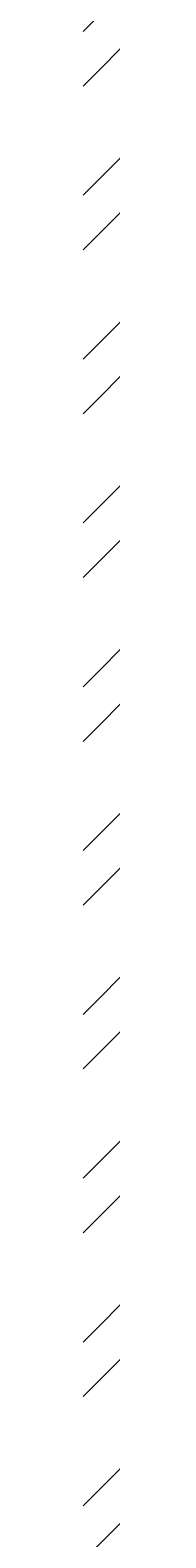
# Model space of a CAD drawing. Units: inches. Extents: x 1962 to 2771, y 1245 to 2660.
# Tile 106 of 114: x 2372 to 2374, y 2180 to 2304. Entities that reach past the tile are written whole.
import ezdxf

# ---------------------------------------------------------------- set-up
doc = ezdxf.new("R2010")
doc.units = ezdxf.units.IN
doc.layers.add('A-ANNO-DIMS', color=2, linetype='Continuous', lineweight=18)
doc.layers.add('A-WALL-PATT', color=252, linetype='Continuous', lineweight=13)
doc.styles.get("Standard").update_dxf_attribs({"font": 'arial.ttf'})
doc.dimstyles.get("Standard").update_dxf_attribs({"dimtxt": 0.18, "dimasz": 0.18, "dimexe": 0.18, "dimexo": 0.0625, "dimgap": 0.09, "dimtad": 0, "dimtih": 1, "dimtoh": 1, "dimdec": 4, "dimzin": 0, "dimdsep": 46, "dimtxsty": 'Standard', "dimcen": 0.09, "dimadec": 0, "dimazin": 0, "dimtfac": 1, "dimtdec": 4, "dimtofl": 0, "dimtmove": 0, "dimatfit": 3, "dimfxl": 1, "dimtolj": 1, "dimtzin": 0, "dimarcsym": 0})

# ---------------------------------------------------------------- blocks, each defined once
blk = doc.blocks.new('*D40')
at = {"layer": 'A-ANNO-DIMS', "color": 0, "lineweight": -2, "transparency": 16777216}
for p, q in [((2072.02, 2033.91), (2072.02, 2583.47)), ((2660.81, 2524.41), (2660.81, 2583.47)), ((2072.2, 2583.29), (2366.02, 2583.29)), ((2660.63, 2583.29), (2366.81, 2583.29))]:
    blk.add_line(p, q, dxfattribs=at)
at = {"layer": 'A-ANNO-DIMS', "color": 0, "transparency": 16777216}
for points in [[(2072.2, 2583.32), (2072.2, 2583.26), (2072.02, 2583.29)], [(2660.63, 2583.32), (2660.63, 2583.26), (2660.81, 2583.29)]]:
    blk.add_solid(points, dxfattribs=at)
at = {"layer": 'Defpoints', "color": 0, "transparency": 16777216}
for p in [(2660.81, 2583.29), (2660.81, 2524.34), (2072.02, 2033.84)]:
    blk.add_point(p, dxfattribs=at)
at = {"layer": 'A-ANNO-DIMS', "color": 0, "transparency": 16777216, "insert": (2366.41, 2583.29), "char_height": 0.18, "attachment_point": 5}
blk.add_mtext('\\A1;588.8', dxfattribs=at)

msp = doc.modelspace()

# ---------------------------------------------------------------- hatches: boundary and pattern name
at = {"layer": 'A-WALL-PATT'}
h = msp.add_hatch(dxfattribs=at)
h.set_pattern_fill('ANSI32', color=256)
h.paths.add_polyline_path([(2090.8074, 2467.3437), (2141.6481, 2467.3437), (2141.6481, 2469.5937), (2141.6481, 2471.8437), (2086.3074, 2471.8437), (2086.3074, 2422.5333), (2090.8074, 2422.5333)])
h.paths.add_polyline_path([(2282.7664, 2471.8437), (2204.8982, 2471.8437), (2204.8982, 2467.3437), (2234.8074, 2467.3437), (2234.8074, 2311.3437), (2228.7492, 2311.3437), (2228.7492, 2306.8437), (2234.8074, 2306.8437), (2331.9227, 2306.8437), (2331.9227, 2309.0937), (2331.9227, 2311.3437), (2239.3074, 2311.3437), (2239.3074, 2467.3437), (2282.7664, 2467.3437), (2282.7664, 2469.5937)])
h.paths.add_polyline_path([(2471.4531, 2519.8437), (2552.011, 2519.8437), (2564.3996, 2519.8437), (2564.3996, 2511.1389), (2568.8996, 2511.1389), (2568.8996, 2524.3437), (2466.9531, 2524.3437), (2466.9531, 2471.8437), (2450.0749, 2471.8437), (2446.4672, 2471.8437), (2446.4672, 2467.3437), (2450.0749, 2467.3437), (2475.9988, 2467.3437), (2475.9988, 2469.5937), (2475.9988, 2471.8437), (2471.4531, 2471.8437)])
h.paths.add_polyline_path([(2575.2231, 2469.5937), (2575.2231, 2471.8437), (2568.8996, 2471.8437), (2568.8996, 2487.1389), (2564.3996, 2487.1389), (2564.3996, 2471.8437), (2556.511, 2471.8437), (2499.2904, 2471.8437), (2499.2904, 2467.3437), (2507.8074, 2467.3437), (2507.8074, 2311.3437), (2414.863, 2311.3437), (2414.863, 2306.8437), (2512.3074, 2306.8437), (2517.0114, 2306.8437), (2517.0114, 2309.0937), (2517.0114, 2311.3437), (2512.3074, 2311.3437), (2512.3074, 2467.3437), (2575.2231, 2467.3437)])
h.paths.add_polyline_path([(2660.8074, 2471.8437), (2600.9602, 2471.8437), (2600.9602, 2467.3437), (2656.3074, 2467.3437), (2656.3074, 2432.5704), (2660.8074, 2432.5704)])
h.paths.add_polyline_path([(2660.8074, 2372.5704), (2656.3074, 2372.5704), (2656.3074, 2311.3437), (2600.276, 2311.3437), (2600.276, 2309.0937), (2600.276, 2306.8437), (2656.3074, 2306.8437), (2656.3074, 2296.2593), (2660.8074, 2296.2593)])
h.paths.add_polyline_path([(2572.3074, 2306.8437), (2577.1385, 2306.8437), (2577.1385, 2311.3437), (2551.082, 2311.3437), (2551.082, 2306.8437), (2567.8074, 2306.8437), (2567.8074, 2258.8437), (2540.0574, 2258.8437), (2540.0574, 2256.5937), (2540.0574, 2254.3437), (2567.8074, 2254.3437), (2656.3074, 2254.3437), (2656.3074, 2236.9085), (2660.8074, 2236.9085), (2660.8074, 2272.2593), (2656.3074, 2272.2593), (2656.3074, 2258.8437), (2572.3074, 2258.8437)])
h.paths.add_polyline_path([(2512.3074, 2254.3437), (2518.8716, 2254.3437), (2518.8716, 2256.5937), (2518.8716, 2258.8437), (2507.8074, 2258.8437), (2507.8074, 2177.8437), (2567.8074, 2177.8437), (2567.8074, 2172.9628), (2572.3074, 2172.9628), (2572.3074, 2177.8437), (2656.3074, 2177.8437), (2656.3074, 2166.4846), (2660.8074, 2166.4846), (2660.8074, 2200.9085), (2656.3074, 2200.9085), (2656.3074, 2182.3437), (2512.3074, 2182.3437)])
h.paths.add_polyline_path([(2656.3074, 2129.8437), (2572.3074, 2129.8437), (2572.3074, 2150.3044), (2570.0574, 2150.3044), (2567.8074, 2150.3044), (2567.8074, 2129.8437), (2507.8074, 2129.8437), (2507.8074, 2116.3027), (2510.0574, 2116.3027), (2512.3074, 2116.3027), (2512.3074, 2125.3437), (2567.8074, 2125.3437), (2572.3074, 2125.3437), (2656.3074, 2125.3437)])
h.paths.add_polyline_path([(2090.8074, 2362.5333), (2086.3074, 2362.5333), (2086.3074, 2298.6242), (2090.8074, 2298.6242), (2090.8074, 2306.8437), (2174.8074, 2306.8437), (2174.8074, 2286.4178), (2179.3074, 2286.4178), (2179.3074, 2306.8437), (2192.8641, 2306.8437), (2192.8641, 2309.0937), (2192.8641, 2311.3437), (2090.8074, 2311.3437)])
h.paths.add_polyline_path([(2209.156, 2258.8437), (2179.3074, 2258.8437), (2179.3074, 2263.2236), (2177.0574, 2263.2236), (2174.8074, 2263.2236), (2174.8074, 2258.8437), (2090.8074, 2258.8437), (2090.8074, 2274.6242), (2086.3074, 2274.6242), (2086.3074, 2238.2967), (2088.5574, 2238.2967), (2090.8074, 2238.2967), (2090.8074, 2254.3437), (2209.156, 2254.3437)])
h.paths.add_polyline_path([(2090.8074, 2177.8437), (2234.8074, 2177.8437), (2234.8074, 2173.1428), (2239.3074, 2173.1428), (2239.3074, 2258.8437), (2230.8442, 2258.8437), (2230.8442, 2256.5937), (2230.8442, 2254.3437), (2234.8074, 2254.3437), (2234.8074, 2182.3437), (2090.8074, 2182.3437), (2090.8074, 2202.2967), (2086.3074, 2202.2967), (2086.3074, 2140.0389), (2090.8074, 2140.0389)])
h.paths.add_polyline_path([(2090.8074, 2080.0389), (2086.3074, 2080.0389), (2086.3074, 2033.8437), (2090.8074, 2033.8437)], flags=17)
h.paths.add_polyline_path([(2244.9405, 2033.8437), (2239.3074, 2033.8437), (2239.3074, 2142.0665), (2237.2592, 2142.0665), (2234.8074, 2142.0665), (2234.8074, 2033.8437), (2090.8074, 2033.8437), (2076.5204, 2033.8437), (2072.0204, 2033.8437), (2072.0204, 2000.4493), (2076.5204, 2000.4493), (2076.5204, 2029.3437), (2090.8074, 2029.3437), (2244.9405, 2029.3437), (2244.9405, 2031.5937)])
h.paths.add_polyline_path([(2234.8074, 1933.3437), (2076.5204, 1933.3437), (2076.5204, 1952.4493), (2074.2704, 1952.4493), (2072.0204, 1952.4493), (2072.0204, 1933.3437), (2072.0204, 1928.8437), (2234.8074, 1928.8437)])
h.paths.add_polyline_path([(2090.8074, 1928.8437), (2086.3074, 1928.8437), (2086.3074, 1906.5013), (2090.8074, 1906.5013)])
h.paths.add_polyline_path([(2090.8074, 1846.5013), (2086.3074, 1846.5013), (2086.3074, 1769.9917), (2088.5574, 1769.9917), (2090.8074, 1769.9917), (2090.8074, 1780.3437), (2234.8074, 1780.3437), (2234.8074, 1708.3437), (2230.3764, 1708.3437), (2230.3764, 1703.8437), (2239.3074, 1703.8437), (2239.3074, 1792.6669), (2237.0574, 1792.6669), (2234.8074, 1792.6669), (2234.8074, 1784.8437), (2090.8074, 1784.8437)])
h.paths.add_polyline_path([(2239.3074, 1928.8437), (2244.9405, 1928.8437), (2244.9405, 1931.0937), (2244.9405, 1933.3437), (2234.8074, 1933.3437), (2234.8074, 1928.8437), (2234.8074, 1825.5949), (2239.3074, 1825.5949)])
h.paths.add_polyline_path([(2148.0425, 1649.0937), (2148.0425, 1651.3437), (2090.8074, 1651.3437), (2090.8074, 1646.8437), (2148.0425, 1646.8437)], flags=0)
h.paths.add_polyline_path([(2207.5601, 1708.3437), (2090.8074, 1708.3437), (2090.8074, 1703.8437), (2174.8074, 1703.8437), (2174.8074, 1651.3437), (2170.4457, 1651.3437), (2170.4457, 1646.8437), (2195.9924, 1646.8437), (2195.9924, 1649.0937), (2195.9924, 1651.3437), (2179.3074, 1651.3437), (2179.3074, 1703.8437), (2207.5601, 1703.8437), (2207.5601, 1706.0937)])
h.paths.add_polyline_path([(2090.8074, 1733.9917), (2086.3074, 1733.9917), (2086.3074, 1696.1032), (2088.5574, 1696.1032), (2090.8074, 1696.1032)])
h.paths.add_polyline_path([(2090.8074, 1672.1032), (2086.3074, 1672.1032), (2086.3074, 1600.3335), (2090.8074, 1600.3335)])
h.paths.add_polyline_path([(2090.8074, 1540.3335), (2086.3074, 1540.3335), (2086.3074, 1486.3437), (2139.6766, 1486.3437), (2139.6766, 1490.8437), (2090.8074, 1490.8437)])
h.paths.add_polyline_path([(2302.3876, 1490.8437), (2239.3074, 1490.8437), (2239.3074, 1646.8437), (2335.9994, 1646.8437), (2335.9994, 1651.3437), (2229.884, 1651.3437), (2229.884, 1646.8437), (2234.8074, 1646.8437), (2234.8074, 1490.8437), (2202.7103, 1490.8437), (2202.7103, 1488.5937), (2202.7103, 1486.3437), (2275.0699, 1486.3437), (2275.0699, 1475.772), (2279.5699, 1475.772), (2279.5699, 1486.3437), (2302.3876, 1486.3437)])
h.paths.add_polyline_path([(2279.5699, 1451.772), (2275.0699, 1451.772), (2275.0699, 1438.3437), (2174.8074, 1438.3437), (2174.8074, 1486.3437), (2179.7922, 1486.3437), (2179.7922, 1490.8437), (2163.3585, 1490.8437), (2163.3585, 1488.5937), (2163.3585, 1486.3437), (2170.3074, 1486.3437), (2170.3074, 1433.8437), (2279.5699, 1433.8437)])
h.paths.add_polyline_path([(2427.2363, 1490.8437), (2375.8074, 1490.8437), (2375.8074, 1646.8437), (2381.6401, 1646.8437), (2381.6401, 1651.3437), (2365.887, 1651.3437), (2365.887, 1649.0937), (2365.887, 1646.8437), (2371.3074, 1646.8437), (2371.3074, 1490.8437), (2327.5627, 1490.8437), (2327.5627, 1488.5937), (2327.5627, 1486.3437), (2371.3074, 1486.3437), (2371.3074, 1433.8437), (2375.8074, 1433.8437), (2375.8074, 1486.3437), (2427.2363, 1486.3437)])
h.paths.add_polyline_path([(2512.3074, 1646.8437), (2519.4351, 1646.8437), (2519.4351, 1649.0937), (2519.4351, 1651.3437), (2507.8074, 1651.3437), (2416.0063, 1651.3437), (2416.0063, 1649.0937), (2416.0063, 1646.8437), (2507.8074, 1646.8437), (2507.8074, 1490.8437), (2497.0532, 1490.8437), (2497.0532, 1488.5937), (2497.0532, 1486.3437), (2574.9344, 1486.3437), (2574.9344, 1476.0181), (2579.4344, 1476.0181), (2579.4344, 1486.3437), (2584.4872, 1486.3437), (2584.3074, 1490.8437), (2512.3074, 1490.8437)])
h.paths.add_polyline_path([(2470.5091, 1486.3437), (2473.9767, 1486.3437), (2473.9767, 1490.8437), (2449.6605, 1490.8437), (2449.6605, 1488.5937), (2449.6605, 1486.3437), (2466.0091, 1486.3437), (2466.0091, 1433.8437), (2470.5091, 1433.8437), (2579.4344, 1433.8437), (2579.4344, 1452.0181), (2574.9344, 1452.0181), (2574.9344, 1438.3437), (2554.5091, 1438.3437), (2470.5091, 1438.3437)])
h.paths.add_polyline_path([(2656.3074, 1490.8437), (2611.86, 1490.8437), (2611.86, 1486.3437), (2656.3074, 1486.3437)])
h.paths.add_polyline_path([(2660.8074, 1532.7007), (2658.5574, 1532.7007), (2656.3074, 1532.7007), (2656.3074, 1486.3437), (2660.8074, 1486.3437)])
h.paths.add_polyline_path([(2660.8074, 1664.9663), (2656.3074, 1664.9663), (2656.3074, 1651.3437), (2602.2313, 1651.3437), (2602.2313, 1646.8437), (2656.3074, 1646.8437), (2656.3074, 1592.7007), (2660.8074, 1592.7007)])
h.paths.add_polyline_path([(2660.8074, 1724.5221), (2656.3074, 1724.5221), (2656.3074, 1703.8437), (2542.4725, 1703.8437), (2542.4725, 1699.3437), (2567.8074, 1699.3437), (2567.8074, 1651.3437), (2552.7766, 1651.3437), (2552.7766, 1649.0937), (2552.7766, 1646.8437), (2577.2878, 1646.8437), (2577.2878, 1649.0937), (2577.2878, 1651.3437), (2572.3074, 1651.3437), (2572.3074, 1699.3437), (2656.3074, 1699.3437), (2656.3074, 1688.9663), (2660.8074, 1688.9663)])
h.paths.add_polyline_path([(2660.8074, 1880.6524), (2656.3074, 1880.6524), (2656.3074, 1832.8437), (2512.3074, 1832.8437), (2512.3074, 1837.8959), (2507.8074, 1837.8959), (2507.8074, 1828.3437), (2567.8074, 1828.3437), (2567.8074, 1804.3437), (2572.3074, 1804.3437), (2572.3074, 1828.3437), (2656.3074, 1828.3437), (2656.3074, 1818.6778), (2660.8074, 1818.6778)])
h.paths.add_polyline_path([(2660.8074, 1794.6778), (2656.3074, 1794.6778), (2656.3074, 1780.3437), (2572.3074, 1780.3437), (2572.3074, 1783.0303), (2570.0574, 1783.0303), (2567.8074, 1783.0303), (2567.8074, 1780.3437), (2507.8074, 1780.3437), (2507.8074, 1699.3437), (2517.8858, 1699.3437), (2517.8858, 1701.5937), (2517.8858, 1703.8437), (2512.3074, 1703.8437), (2512.3074, 1775.8437), (2656.3074, 1775.8437), (2656.3074, 1760.5221), (2660.8074, 1760.5221)])
h.paths.add_polyline_path([(2660.8074, 1981.3437), (2660.8074, 2020.2808), (2658.5574, 2020.2808), (2656.3074, 2020.2808), (2656.3074, 1981.3437), (2512.3074, 1981.3437), (2512.3074, 2086.6996), (2507.8074, 2086.6996), (2507.8074, 1981.3437), (2375.8074, 1981.3437), (2375.8074, 1986.8505), (2373.5574, 1986.8505), (2371.3074, 1986.8505), (2371.3074, 1973.2607), (2375.8074, 1973.2607), (2375.8074, 1976.8437), (2507.8074, 1976.8437), (2507.8074, 1865.4281), (2510.0574, 1865.4281), (2512.3074, 1865.4281), (2512.3074, 1976.8437), (2660.8074, 1976.8437)])
h.paths.add_polyline_path([(2375.8074, 1940.297), (2373.5574, 1940.297), (2371.3074, 1940.297), (2371.3074, 1933.3437), (2278.4434, 1933.3437), (2278.4434, 1928.8437), (2371.3074, 1928.8437), (2371.3074, 1651.3437), (2375.8074, 1651.3437)])
h.paths.add_polyline_path([(2660.8074, 1976.8437), (2656.3074, 1976.8437), (2656.3074, 1940.6524), (2660.8074, 1940.6524)], flags=17)
h.paths.add_polyline_path([(2660.8074, 2142.4846), (2656.3074, 2142.4846), (2656.3074, 2080.2808), (2660.8074, 2080.2808)])
h.paths.add_polyline_path([(2381.4189, 2311.3437), (2375.8074, 2311.3437), (2375.8074, 2467.3437), (2424.7242, 2467.3437), (2424.7242, 2469.5937), (2424.7242, 2471.8437), (2375.8074, 2471.8437), (2375.8074, 2524.3437), (2371.3074, 2524.3437), (2371.3074, 2471.8437), (2307.2097, 2471.8437), (2307.2097, 2467.3437), (2371.3074, 2467.3437), (2371.3074, 2311.3437), (2366.8901, 2311.3437), (2366.8901, 2306.8437), (2371.3074, 2306.8437), (2371.3074, 2033.8437), (2279.6589, 2033.8437), (2279.6589, 2029.3437), (2371.3074, 2029.3437), (2371.3074, 2014.2598), (2375.8074, 2014.2598), (2375.8074, 2306.8437), (2381.4189, 2306.8437)])
h.paths.add_polyline_path([(2263.3074, 2524.3437), (2170.3074, 2524.3437), (2170.3074, 2519.8437), (2170.3074, 2471.8437), (2165.0312, 2471.8437), (2165.0312, 2467.3437), (2179.6721, 2467.3437), (2179.6721, 2469.5161), (2179.6721, 2471.8437), (2174.8074, 2471.8437), (2174.8074, 2519.8437), (2258.8074, 2519.8437), (2258.8074, 2511.6436), (2263.3074, 2511.6436)])
h.paths.add_polyline_path([(2245.0232, 1361.4123), (2492.9468, 1361.4123), (2492.9468, 1398.505), (2245.0232, 1398.505)], flags=9)
h.paths.add_polyline_path([(2388.1434, 2086.6936), (2425.0704, 2086.6936), (2425.0704, 2105.3509), (2388.1434, 2105.3509)], flags=9)
h.paths.add_polyline_path([(2404.922, 2242.6744), (2445.7337, 2242.6744), (2445.7337, 2261.3318), (2404.922, 2261.3318)], flags=9)
h.paths.add_polyline_path([(2269.4107, 2156.7935), (2306.3378, 2156.7935), (2306.3378, 2175.4508), (2269.4107, 2175.4508)], flags=9)
h.paths.add_polyline_path([(2269.3277, 2233.4343), (2306.2547, 2233.4343), (2306.2547, 2252.0917), (2269.3277, 2252.0917)], flags=9)
h.paths.add_polyline_path([(2431.6052, 2320.6922), (2470.4456, 2320.6922), (2470.4456, 2339.3495), (2431.6052, 2339.3495)], flags=25)
h.paths.add_polyline_path([(2249.6902, 2315.7608), (2288.5306, 2315.7608), (2288.5306, 2334.4182), (2249.6902, 2334.4182)], flags=25)
h.paths.add_polyline_path([(2096.9301, 2314.3181), (2135.7704, 2314.3181), (2135.7704, 2332.9755), (2096.9301, 2332.9755)], flags=25)
h.paths.add_polyline_path([(2134.3475, 2285.7089), (2161.4655, 2285.7089), (2161.4655, 2304.3662), (2134.3475, 2304.3662)], flags=9)
h.paths.add_polyline_path([(2126.5155, 2209.4076), (2159.9227, 2209.4076), (2159.9227, 2228.065), (2126.5155, 2228.065)], flags=25)
h.paths.add_polyline_path([(2110.5753, 2141.5299), (2149.4157, 2141.5299), (2149.4157, 2160.1872), (2110.5753, 2160.1872)], flags=25)
h.paths.add_polyline_path([(2249.8618, 1968.3317), (2286.3966, 1968.3317), (2286.3966, 1986.989), (2249.8618, 1986.989)], flags=9)
h.paths.add_polyline_path([(2395.9507, 1777.0051), (2436.7624, 1777.0051), (2436.7624, 1795.6625), (2395.9507, 1795.6625)], flags=9)
h.paths.add_polyline_path([(2398.5259, 1888.5651), (2435.0062, 1888.5651), (2435.0062, 1907.2224), (2398.5259, 1907.2224)], flags=25)
h.paths.add_polyline_path([(2259.3506, 1728.3559), (2296.2776, 1728.3559), (2296.2776, 1747.0132), (2259.3506, 1747.0132)], flags=9)
h.paths.add_polyline_path([(2271.3698, 1845.268), (2308.2968, 1845.268), (2308.2968, 1863.9253), (2271.3698, 1863.9253)], flags=9)
h.paths.add_polyline_path([(2120.9355, 1786.3027), (2159.7759, 1786.3027), (2159.7759, 1804.9601), (2120.9355, 1804.9601)], flags=25)
h.paths.add_polyline_path([(2121.3164, 1732.1043), (2154.7236, 1732.1043), (2154.7236, 1750.7616), (2121.3164, 1750.7616)], flags=25)
h.paths.add_polyline_path([(2118.3706, 1678.8997), (2147.5282, 1678.8997), (2147.5282, 1697.557), (2118.3706, 1697.557)], flags=25)
h.paths.add_polyline_path([(2385.9227, 1493.557), (2424.763, 1493.557), (2424.763, 1512.2143), (2385.9227, 1512.2143)], flags=25)
h.paths.add_polyline_path([(2248.7058, 1500.0256), (2287.5462, 1500.0256), (2287.5462, 1518.6829), (2248.7058, 1518.6829)], flags=25)
h.paths.add_polyline_path([(2104.1669, 1617.3771), (2143.0073, 1617.3771), (2143.0073, 1636.0344), (2104.1669, 1636.0344)], flags=9)
h.paths.add_polyline_path([(2096.0714, 1447.8824), (2137.3845, 1447.8824), (2137.3845, 1458.1859), (2096.0714, 1458.1859)], flags=9)
h.paths.add_polyline_path([(2180.6114, 1440.325), (2209.7689, 1440.325), (2209.7689, 1458.9823), (2180.6114, 1458.9823)], flags=25)
h.paths.add_polyline_path([(2316.1698, 1447.9637), (2357.4829, 1447.9637), (2357.4829, 1458.2673), (2316.1698, 1458.2673)], flags=9)
h.paths.add_polyline_path([(2397.6187, 1447.9637), (2438.9318, 1447.9637), (2438.9318, 1458.2673), (2397.6187, 1458.2673)], flags=9)
h.paths.add_polyline_path([(2473.0778, 1439.5953), (2502.2354, 1439.5953), (2502.2354, 1458.2527), (2473.0778, 1458.2527)], flags=25)
h.paths.add_polyline_path([(2589.7027, 1447.8819), (2631.0158, 1447.8819), (2631.0158, 1458.1855), (2589.7027, 1458.1855)], flags=9)
h.paths.add_polyline_path([(2522.4009, 1497.5285), (2561.2413, 1497.5285), (2561.2413, 1516.1859), (2522.4009, 1516.1859)], flags=25)
h.paths.add_polyline_path([(2579.6565, 1671.3482), (2608.8141, 1671.3482), (2608.8141, 1690.0056), (2579.6565, 1690.0056)], flags=25)
h.paths.add_polyline_path([(2544.7038, 1725.5064), (2578.1111, 1725.5064), (2578.1111, 1744.1637), (2544.7038, 1744.1637)], flags=25)
h.paths.add_polyline_path([(2578.1191, 1807.472), (2607.2766, 1807.472), (2607.2766, 1826.1293), (2578.1191, 1826.1293)], flags=25)
h.paths.add_polyline_path([(2595.0614, 1835.1839), (2633.9018, 1835.1839), (2633.9018, 1853.8413), (2595.0614, 1853.8413)], flags=25)
h.paths.add_polyline_path([(2567.0097, 2097.7035), (2605.8501, 2097.7035), (2605.8501, 2116.3609), (2567.0097, 2116.3609)], flags=9)
h.paths.add_polyline_path([(2586.644, 2134.6454), (2615.8015, 2134.6454), (2615.8015, 2153.3027), (2586.644, 2153.3027)], flags=9)
h.paths.add_polyline_path([(2544.6185, 2212.6783), (2578.0258, 2212.6783), (2578.0258, 2231.3356), (2544.6185, 2231.3356)], flags=25)
h.paths.add_polyline_path([(2577.0273, 2256.9023), (2606.1849, 2256.9023), (2606.1849, 2275.5597), (2577.0273, 2275.5597)], flags=24)
h.paths.add_polyline_path([(2605.2683, 2315.2821), (2644.1087, 2315.2821), (2644.1087, 2333.9395), (2605.2683, 2333.9395)], flags=25)
h.paths.add_polyline_path([(2583.1244, 2496.1815), (2624.4375, 2496.1815), (2624.4375, 2506.4851), (2583.1244, 2506.4851)], flags=9)
h.paths.add_polyline_path([(2474.761, 2497.0823), (2503.9185, 2497.0823), (2503.9185, 2515.7397), (2474.761, 2515.7397)], flags=25)
h.paths.add_polyline_path([(2387.5787, 2494.2563), (2428.902, 2494.2563), (2428.902, 2504.5598), (2387.5787, 2504.5598)], flags=9)
h.paths.add_polyline_path([(2300.1657, 2500.1564), (2341.4788, 2500.1564), (2341.4788, 2510.46), (2300.1657, 2510.46)], flags=25)
h.paths.add_polyline_path([(2176.8589, 2497.5843), (2206.0165, 2497.5843), (2206.0165, 2516.2416), (2176.8589, 2516.2416)], flags=25)
h.paths.add_polyline_path([(2097.4668, 2494.9762), (2138.7799, 2494.9762), (2138.7799, 2505.2798), (2097.4668, 2505.2798)], flags=9)

# ---------------------------------------------------------------- dimensions: what is measured, and where the dimension line sits
at = {"layer": 'A-ANNO-DIMS'}
dim = msp.add_linear_dim(base=(2660.8074, 2583.2937), p1=(2072.0204, 2033.8437), p2=(2660.8074, 2524.3437), dimstyle='Standard', override={"dimdec": 1, "dimlfac": 1, "dimrnd": 0, "dimzin": 0, "dimdsep": 46, "dimlunit": 2}, dxfattribs=at)
dim.commit()
dim.dimension.update_dxf_attribs({"geometry": '*D40', "text_midpoint": (2366.4139, 2583.2937)})

doc.saveas('drawing.dxf')
